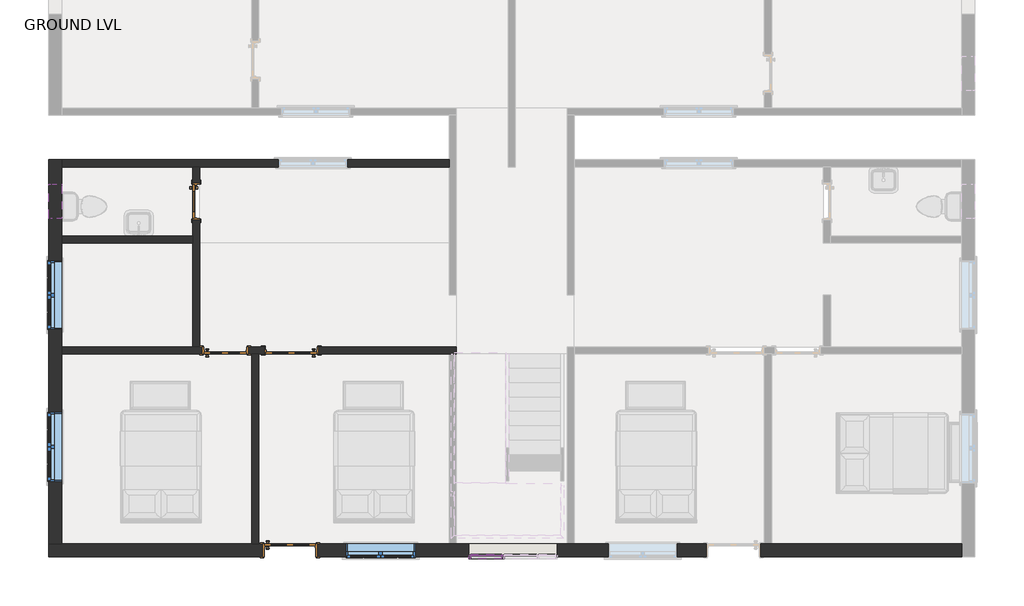
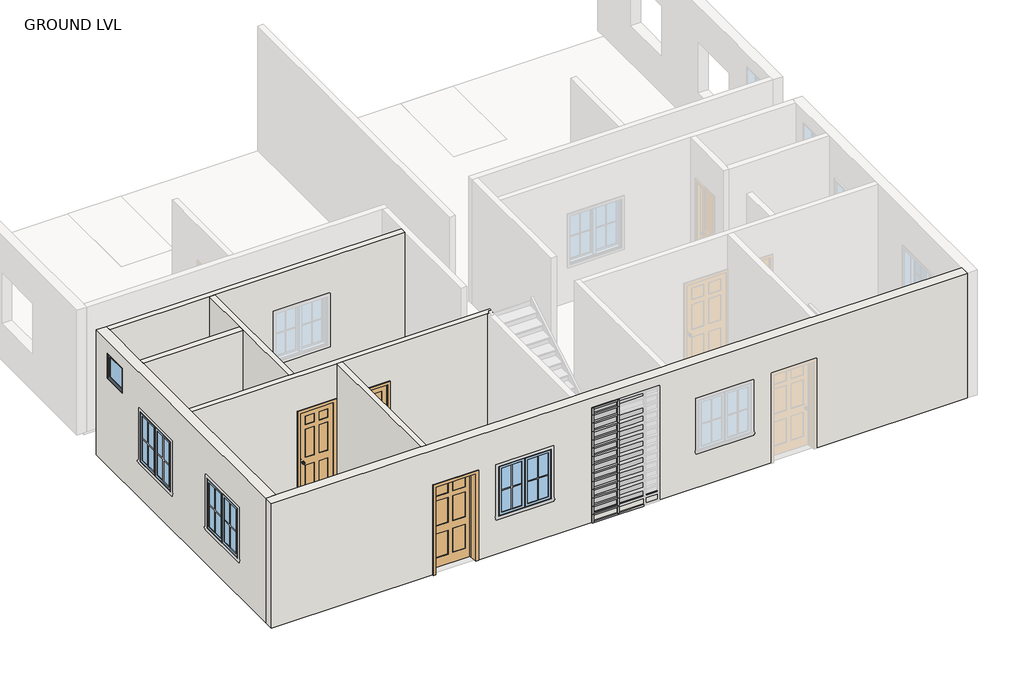
# One storey, part 1 of 4: 44 members, 27 plates, 7 walls, 4 doors, 4 windows.
"""IFC4 building model written with IfcOpenShell, lengths in millimetres."""

from ifc_helpers import new_model, si_unit, origin, origin_with_axes, place, context, project, spatial, polyline, outline, extrude, faceted_brep, transform, mapped, element, save
from components import door_e337afa5, door_3b50870b, door_d86b6c54, door_03e3dfb5, member_56b223d9, member_a59c64b1, member_fa69921b, member_a67f877f, member_6a7c88b6, member_dc11c383, member_ff422208, system_panel_glazed_844a74e3, system_panel_glazed_a39216e9, system_panel_glazed_b3845325, system_panel_glazed_23b8b45c, system_panel_glazed_26c33eb0, system_panel_glazed_afc0885c, window_80340324, window_9200f5ac

model = new_model("IFC4")

# Units and contexts
model_context = context("Model", 3, world=origin())
ifc_project = project(units=[si_unit("LENGTHUNIT", "METRE", prefix="MILLI")], contexts=[model_context])

# Site, building, storey
site = spatial("IfcSite", under=ifc_project)
building = spatial("IfcBuilding", under=site)
storey = spatial("IfcBuildingStorey", under=building, Name="GROUND LVL", Elevation=0.0)

# Doors
placement = place(None, origin())
door_shape = door_e337afa5(model_context)
element("IfcDoor", 1, ObjectType="Door-Interior-Single-2_Panel-Wood : 24\" x 84\"", at=placement, inside=storey, context=model_context, shape_type="MappedRepresentation", body=[
    mapped(door_shape, transform((-9830.0887331, -1548.6593836, 0.0), x_axis=(0.0, -1.0, 0.0), y_axis=(1.0, 0.0, 0.0), z_axis=(0.0, 0.0, 1.0))),
])
door_2_shape = door_3b50870b(model_context)
element("IfcDoor", 2, ObjectType="Door-Interior-Single-6_Panel-Wood : 30\" x 84\"", at=placement, inside=storey, context=model_context, shape_type="MappedRepresentation", body=[
    mapped(door_2_shape, transform((-9318.9137331, -4180.7343836, 0.0), x_axis=(1.0, 0.0, 0.0), y_axis=(0.0, 1.0, 0.0), z_axis=(0.0, 0.0, 1.0))),
])
door_3_shape = door_d86b6c54(model_context)
element("IfcDoor", 3, ObjectType="Door-Interior-Single-6_Panel-Wood : 36\" x 84\"", at=placement, inside=storey, context=model_context, shape_type="MappedRepresentation", body=[
    mapped(door_3_shape, transform((-8175.9137331, -7704.9843836, 0.0), x_axis=(1.0, 0.0, 0.0), y_axis=(0.0, 1.0, 0.0), z_axis=(0.0, 0.0, 1.0))),
])
door_4_shape = door_03e3dfb5(model_context)
element("IfcDoor", 4, ObjectType="Door-Interior-Single-6_Panel-Wood : 36\" x 84\"", at=placement, inside=storey, context=model_context, shape_type="MappedRepresentation", body=[
    mapped(door_4_shape, transform((-8150.5137331, -4180.7343836, 0.0), x_axis=(-1.0, 0.0, 0.0), y_axis=(0.0, -1.0, 0.0), z_axis=(0.0, 0.0, 1.0))),
])

# Members
member_shape = member_56b223d9(model_context)
element("IfcMember", 5, ObjectType="Rectangular Mullion : 1.5\" x 2.5\" rectangular", at=placement, inside=storey, context=model_context, shape_type="MappedRepresentation", body=[
    mapped(member_shape, transform((-4416.6334597, -7822.4593836, 0.0), x_axis=(1.0, 0.0, 0.0), y_axis=(0.0, -1.0, 0.0), z_axis=(0.0, 0.0, -1.0))),
])
element("IfcMember", 6, ObjectType="Rectangular Mullion : 1.5\" x 2.5\" rectangular", at=placement, inside=storey, context=model_context, shape_type="MappedRepresentation", body=[
    mapped(member_shape, transform((-4416.6334597, -7822.4593836, 203.2), x_axis=(1.0, 0.0, 0.0), y_axis=(0.0, -1.0, 0.0), z_axis=(0.0, 0.0, -1.0))),
])
element("IfcMember", 7, ObjectType="Rectangular Mullion : 1.5\" x 2.5\" rectangular", at=placement, inside=storey, context=model_context, shape_type="MappedRepresentation", body=[
    mapped(member_shape, transform((-4416.6334597, -7822.4593836, 406.4), x_axis=(1.0, 0.0, 0.0), y_axis=(0.0, -1.0, 0.0), z_axis=(0.0, 0.0, -1.0))),
])
element("IfcMember", 8, ObjectType="Rectangular Mullion : 1.5\" x 2.5\" rectangular", at=placement, inside=storey, context=model_context, shape_type="MappedRepresentation", body=[
    mapped(member_shape, transform((-4416.6334597, -7822.4593836, 609.6), x_axis=(1.0, 0.0, 0.0), y_axis=(0.0, -1.0, 0.0), z_axis=(0.0, 0.0, -1.0))),
])
element("IfcMember", 9, ObjectType="Rectangular Mullion : 1.5\" x 2.5\" rectangular", at=placement, inside=storey, context=model_context, shape_type="MappedRepresentation", body=[
    mapped(member_shape, transform((-4416.6334597, -7822.4593836, 812.8), x_axis=(1.0, 0.0, 0.0), y_axis=(0.0, -1.0, 0.0), z_axis=(0.0, 0.0, -1.0))),
])
element("IfcMember", 10, ObjectType="Rectangular Mullion : 1.5\" x 2.5\" rectangular", at=placement, inside=storey, context=model_context, shape_type="MappedRepresentation", body=[
    mapped(member_shape, transform((-4416.6334597, -7822.4593836, 1016.0), x_axis=(1.0, 0.0, 0.0), y_axis=(0.0, -1.0, 0.0), z_axis=(0.0, 0.0, -1.0))),
])
element("IfcMember", 11, ObjectType="Rectangular Mullion : 1.5\" x 2.5\" rectangular", at=placement, inside=storey, context=model_context, shape_type="MappedRepresentation", body=[
    mapped(member_shape, transform((-4416.6334597, -7822.4593836, 1219.2), x_axis=(1.0, 0.0, 0.0), y_axis=(0.0, -1.0, 0.0), z_axis=(0.0, 0.0, -1.0))),
])
element("IfcMember", 12, ObjectType="Rectangular Mullion : 1.5\" x 2.5\" rectangular", at=placement, inside=storey, context=model_context, shape_type="MappedRepresentation", body=[
    mapped(member_shape, transform((-4416.6334597, -7822.4593836, 1422.4), x_axis=(1.0, 0.0, 0.0), y_axis=(0.0, -1.0, 0.0), z_axis=(0.0, 0.0, -1.0))),
])
element("IfcMember", 13, ObjectType="Rectangular Mullion : 1.5\" x 2.5\" rectangular", at=placement, inside=storey, context=model_context, shape_type="MappedRepresentation", body=[
    mapped(member_shape, transform((-4416.6334597, -7822.4593836, 1625.6), x_axis=(1.0, 0.0, 0.0), y_axis=(0.0, -1.0, 0.0), z_axis=(0.0, 0.0, -1.0))),
])
element("IfcMember", 14, ObjectType="Rectangular Mullion : 1.5\" x 2.5\" rectangular", at=placement, inside=storey, context=model_context, shape_type="MappedRepresentation", body=[
    mapped(member_shape, transform((-4416.6334597, -7822.4593836, 1828.8), x_axis=(1.0, 0.0, 0.0), y_axis=(0.0, -1.0, 0.0), z_axis=(0.0, 0.0, -1.0))),
])
element("IfcMember", 15, ObjectType="Rectangular Mullion : 1.5\" x 2.5\" rectangular", at=placement, inside=storey, context=model_context, shape_type="MappedRepresentation", body=[
    mapped(member_shape, transform((-4416.6334597, -7822.4593836, 2032.0), x_axis=(1.0, 0.0, 0.0), y_axis=(0.0, -1.0, 0.0), z_axis=(0.0, 0.0, -1.0))),
])
element("IfcMember", 16, ObjectType="Rectangular Mullion : 1.5\" x 2.5\" rectangular", at=placement, inside=storey, context=model_context, shape_type="MappedRepresentation", body=[
    mapped(member_shape, transform((-4416.6334597, -7822.4593836, 2235.2), x_axis=(1.0, 0.0, 0.0), y_axis=(0.0, -1.0, 0.0), z_axis=(0.0, 0.0, -1.0))),
])
element("IfcMember", 17, ObjectType="Rectangular Mullion : 1.5\" x 2.5\" rectangular", at=placement, inside=storey, context=model_context, shape_type="MappedRepresentation", body=[
    mapped(member_shape, transform((-4416.6334597, -7822.4593836, 2438.4), x_axis=(1.0, 0.0, 0.0), y_axis=(0.0, -1.0, 0.0), z_axis=(0.0, 0.0, -1.0))),
])
member_2_shape = member_a59c64b1(model_context)
element("IfcMember", 18, ObjectType="Rectangular Mullion : 1.5\" x 2.5\" rectangular", at=placement, inside=storey, context=model_context, shape_type="MappedRepresentation", body=[
    mapped(member_2_shape, transform((-4416.6334597, -7822.4593836, 2641.6), x_axis=(1.0, 0.0, 0.0), y_axis=(0.0, -1.0, 0.0), z_axis=(0.0, 0.0, -1.0))),
])
member_3_shape = member_fa69921b(model_context)
element("IfcMember", 19, ObjectType="Rectangular Mullion : 1.5\" x 2.5\" rectangular", at=placement, inside=storey, context=model_context, shape_type="MappedRepresentation", body=[
    mapped(member_3_shape, transform((-4435.6834597, -7822.4593836, 2807.3826151), x_axis=(0.0, 0.0, 1.0), y_axis=(0.0, -1.0, 0.0), z_axis=(1.0, 0.0, 0.0))),
])
element("IfcMember", 20, ObjectType="Rectangular Mullion : 1.5\" x 2.5\" rectangular", at=placement, inside=storey, context=model_context, shape_type="MappedRepresentation", body=[
    mapped(member_3_shape, transform((-4988.13346, -7822.4593836, 0.0), x_axis=(0.0, 0.0, -1.0), y_axis=(0.0, -1.0, 0.0), z_axis=(-1.0, 0.0, 0.0))),
])
member_4_shape = member_a67f877f(model_context)
element("IfcMember", 21, ObjectType="Rectangular Mullion : 1.5\" x 2.5\" rectangular", at=placement, inside=storey, context=model_context, shape_type="MappedRepresentation", body=[
    mapped(member_4_shape, transform((-4397.5834597, -7822.4593836, 0.0), x_axis=(0.0, 0.0, -1.0), y_axis=(0.0, -1.0, 0.0), z_axis=(-1.0, 0.0, 0.0))),
])
member_5_shape = member_6a7c88b6(model_context)
element("IfcMember", 22, ObjectType="Rectangular Mullion : 1.5\" x 2.5\" rectangular", at=placement, inside=storey, context=model_context, shape_type="MappedRepresentation", body=[
    mapped(member_5_shape, transform((-4435.6834597, -7822.4593836, 203.2), x_axis=(0.0, 0.0, 1.0), y_axis=(0.0, -1.0, 0.0), z_axis=(1.0, 0.0, 0.0))),
])
element("IfcMember", 23, ObjectType="Rectangular Mullion : 1.5\" x 2.5\" rectangular", at=placement, inside=storey, context=model_context, shape_type="MappedRepresentation", body=[
    mapped(member_5_shape, transform((-4435.6834597, -7822.4593836, 406.4), x_axis=(0.0, 0.0, 1.0), y_axis=(0.0, -1.0, 0.0), z_axis=(1.0, 0.0, 0.0))),
])
element("IfcMember", 24, ObjectType="Rectangular Mullion : 1.5\" x 2.5\" rectangular", at=placement, inside=storey, context=model_context, shape_type="MappedRepresentation", body=[
    mapped(member_5_shape, transform((-4435.6834597, -7822.4593836, 609.6), x_axis=(0.0, 0.0, 1.0), y_axis=(0.0, -1.0, 0.0), z_axis=(1.0, 0.0, 0.0))),
])
element("IfcMember", 25, ObjectType="Rectangular Mullion : 1.5\" x 2.5\" rectangular", at=placement, inside=storey, context=model_context, shape_type="MappedRepresentation", body=[
    mapped(member_5_shape, transform((-4435.6834597, -7822.4593836, 812.8), x_axis=(0.0, 0.0, 1.0), y_axis=(0.0, -1.0, 0.0), z_axis=(1.0, 0.0, 0.0))),
])
element("IfcMember", 26, ObjectType="Rectangular Mullion : 1.5\" x 2.5\" rectangular", at=placement, inside=storey, context=model_context, shape_type="MappedRepresentation", body=[
    mapped(member_5_shape, transform((-4435.6834597, -7822.4593836, 1016.0), x_axis=(0.0, 0.0, 1.0), y_axis=(0.0, -1.0, 0.0), z_axis=(1.0, 0.0, 0.0))),
])
element("IfcMember", 27, ObjectType="Rectangular Mullion : 1.5\" x 2.5\" rectangular", at=placement, inside=storey, context=model_context, shape_type="MappedRepresentation", body=[
    mapped(member_5_shape, transform((-4435.6834597, -7822.4593836, 1219.2), x_axis=(0.0, 0.0, 1.0), y_axis=(0.0, -1.0, 0.0), z_axis=(1.0, 0.0, 0.0))),
])
element("IfcMember", 28, ObjectType="Rectangular Mullion : 1.5\" x 2.5\" rectangular", at=placement, inside=storey, context=model_context, shape_type="MappedRepresentation", body=[
    mapped(member_5_shape, transform((-4435.6834597, -7822.4593836, 1422.4), x_axis=(0.0, 0.0, 1.0), y_axis=(0.0, -1.0, 0.0), z_axis=(1.0, 0.0, 0.0))),
])
element("IfcMember", 29, ObjectType="Rectangular Mullion : 1.5\" x 2.5\" rectangular", at=placement, inside=storey, context=model_context, shape_type="MappedRepresentation", body=[
    mapped(member_5_shape, transform((-4435.6834597, -7822.4593836, 1625.6), x_axis=(0.0, 0.0, 1.0), y_axis=(0.0, -1.0, 0.0), z_axis=(1.0, 0.0, 0.0))),
])
element("IfcMember", 30, ObjectType="Rectangular Mullion : 1.5\" x 2.5\" rectangular", at=placement, inside=storey, context=model_context, shape_type="MappedRepresentation", body=[
    mapped(member_5_shape, transform((-4435.6834597, -7822.4593836, 1828.8), x_axis=(0.0, 0.0, 1.0), y_axis=(0.0, -1.0, 0.0), z_axis=(1.0, 0.0, 0.0))),
])
element("IfcMember", 31, ObjectType="Rectangular Mullion : 1.5\" x 2.5\" rectangular", at=placement, inside=storey, context=model_context, shape_type="MappedRepresentation", body=[
    mapped(member_5_shape, transform((-4435.6834597, -7822.4593836, 2032.0), x_axis=(0.0, 0.0, 1.0), y_axis=(0.0, -1.0, 0.0), z_axis=(1.0, 0.0, 0.0))),
])
element("IfcMember", 32, ObjectType="Rectangular Mullion : 1.5\" x 2.5\" rectangular", at=placement, inside=storey, context=model_context, shape_type="MappedRepresentation", body=[
    mapped(member_5_shape, transform((-4435.6834597, -7822.4593836, 2235.2), x_axis=(0.0, 0.0, 1.0), y_axis=(0.0, -1.0, 0.0), z_axis=(1.0, 0.0, 0.0))),
])
element("IfcMember", 33, ObjectType="Rectangular Mullion : 1.5\" x 2.5\" rectangular", at=placement, inside=storey, context=model_context, shape_type="MappedRepresentation", body=[
    mapped(member_5_shape, transform((-4435.6834597, -7822.4593836, 2438.4), x_axis=(0.0, 0.0, 1.0), y_axis=(0.0, -1.0, 0.0), z_axis=(1.0, 0.0, 0.0))),
])
element("IfcMember", 34, ObjectType="Rectangular Mullion : 1.5\" x 2.5\" rectangular", at=placement, inside=storey, context=model_context, shape_type="MappedRepresentation", body=[
    mapped(member_5_shape, transform((-4435.6834597, -7822.4593836, 2641.6), x_axis=(0.0, 0.0, 1.0), y_axis=(0.0, -1.0, 0.0), z_axis=(1.0, 0.0, 0.0))),
])
member_6_shape = member_dc11c383(model_context)
element("IfcMember", 35, ObjectType="Rectangular Mullion : 1.5\" x 2.5\" rectangular", at=placement, inside=storey, context=model_context, shape_type="MappedRepresentation", body=[
    mapped(member_6_shape, transform((-5026.23346, -7822.4593836, 2807.3826151), x_axis=(-1.0, 0.0, 0.0), y_axis=(0.0, -1.0, 0.0), z_axis=(0.0, 0.0, 1.0))),
])
member_7_shape = member_ff422208(model_context)
element("IfcMember", 36, ObjectType="Rectangular Mullion : 1.5\" x 2.5\" rectangular", at=placement, inside=storey, context=model_context, shape_type="MappedRepresentation", body=[
    mapped(member_7_shape, transform((-5026.23346, -7822.4593836, 203.2), x_axis=(-1.0, 0.0, 0.0), y_axis=(0.0, -1.0, 0.0), z_axis=(0.0, 0.0, 1.0))),
])
element("IfcMember", 37, ObjectType="Rectangular Mullion : 1.5\" x 2.5\" rectangular", at=placement, inside=storey, context=model_context, shape_type="MappedRepresentation", body=[
    mapped(member_7_shape, transform((-5026.23346, -7822.4593836, 406.4), x_axis=(-1.0, 0.0, 0.0), y_axis=(0.0, -1.0, 0.0), z_axis=(0.0, 0.0, 1.0))),
])
element("IfcMember", 38, ObjectType="Rectangular Mullion : 1.5\" x 2.5\" rectangular", at=placement, inside=storey, context=model_context, shape_type="MappedRepresentation", body=[
    mapped(member_7_shape, transform((-5026.23346, -7822.4593836, 609.6), x_axis=(-1.0, 0.0, 0.0), y_axis=(0.0, -1.0, 0.0), z_axis=(0.0, 0.0, 1.0))),
])
element("IfcMember", 39, ObjectType="Rectangular Mullion : 1.5\" x 2.5\" rectangular", at=placement, inside=storey, context=model_context, shape_type="MappedRepresentation", body=[
    mapped(member_7_shape, transform((-5026.23346, -7822.4593836, 812.8), x_axis=(-1.0, 0.0, 0.0), y_axis=(0.0, -1.0, 0.0), z_axis=(0.0, 0.0, 1.0))),
])
element("IfcMember", 40, ObjectType="Rectangular Mullion : 1.5\" x 2.5\" rectangular", at=placement, inside=storey, context=model_context, shape_type="MappedRepresentation", body=[
    mapped(member_7_shape, transform((-5026.23346, -7822.4593836, 1016.0), x_axis=(-1.0, 0.0, 0.0), y_axis=(0.0, -1.0, 0.0), z_axis=(0.0, 0.0, 1.0))),
])
element("IfcMember", 41, ObjectType="Rectangular Mullion : 1.5\" x 2.5\" rectangular", at=placement, inside=storey, context=model_context, shape_type="MappedRepresentation", body=[
    mapped(member_7_shape, transform((-5026.23346, -7822.4593836, 1219.2), x_axis=(-1.0, 0.0, 0.0), y_axis=(0.0, -1.0, 0.0), z_axis=(0.0, 0.0, 1.0))),
])
element("IfcMember", 42, ObjectType="Rectangular Mullion : 1.5\" x 2.5\" rectangular", at=placement, inside=storey, context=model_context, shape_type="MappedRepresentation", body=[
    mapped(member_7_shape, transform((-5026.23346, -7822.4593836, 1422.4), x_axis=(-1.0, 0.0, 0.0), y_axis=(0.0, -1.0, 0.0), z_axis=(0.0, 0.0, 1.0))),
])
element("IfcMember", 43, ObjectType="Rectangular Mullion : 1.5\" x 2.5\" rectangular", at=placement, inside=storey, context=model_context, shape_type="MappedRepresentation", body=[
    mapped(member_7_shape, transform((-5026.23346, -7822.4593836, 1625.6), x_axis=(-1.0, 0.0, 0.0), y_axis=(0.0, -1.0, 0.0), z_axis=(0.0, 0.0, 1.0))),
])
element("IfcMember", 44, ObjectType="Rectangular Mullion : 1.5\" x 2.5\" rectangular", at=placement, inside=storey, context=model_context, shape_type="MappedRepresentation", body=[
    mapped(member_7_shape, transform((-5026.23346, -7822.4593836, 1828.8), x_axis=(-1.0, 0.0, 0.0), y_axis=(0.0, -1.0, 0.0), z_axis=(0.0, 0.0, 1.0))),
])
element("IfcMember", 45, ObjectType="Rectangular Mullion : 1.5\" x 2.5\" rectangular", at=placement, inside=storey, context=model_context, shape_type="MappedRepresentation", body=[
    mapped(member_7_shape, transform((-5026.23346, -7822.4593836, 2032.0), x_axis=(-1.0, 0.0, 0.0), y_axis=(0.0, -1.0, 0.0), z_axis=(0.0, 0.0, 1.0))),
])
element("IfcMember", 46, ObjectType="Rectangular Mullion : 1.5\" x 2.5\" rectangular", at=placement, inside=storey, context=model_context, shape_type="MappedRepresentation", body=[
    mapped(member_7_shape, transform((-5026.23346, -7822.4593836, 2235.2), x_axis=(-1.0, 0.0, 0.0), y_axis=(0.0, -1.0, 0.0), z_axis=(0.0, 0.0, 1.0))),
])
element("IfcMember", 47, ObjectType="Rectangular Mullion : 1.5\" x 2.5\" rectangular", at=placement, inside=storey, context=model_context, shape_type="MappedRepresentation", body=[
    mapped(member_7_shape, transform((-5026.23346, -7822.4593836, 2438.4), x_axis=(-1.0, 0.0, 0.0), y_axis=(0.0, -1.0, 0.0), z_axis=(0.0, 0.0, 1.0))),
])
element("IfcMember", 48, ObjectType="Rectangular Mullion : 1.5\" x 2.5\" rectangular", at=placement, inside=storey, context=model_context, shape_type="MappedRepresentation", body=[
    mapped(member_7_shape, transform((-5026.23346, -7822.4593836, 2641.6), x_axis=(-1.0, 0.0, 0.0), y_axis=(0.0, -1.0, 0.0), z_axis=(0.0, 0.0, 1.0))),
])

# Plates
system_panel_glazed_shape = system_panel_glazed_844a74e3(model_context)
element("IfcPlate", 49, ObjectType="System Panel : Glazed", at=placement, inside=storey, context=model_context, shape_type="MappedRepresentation", body=[
    mapped(system_panel_glazed_shape, transform((-4711.9084599, -7822.4593836, 38.1), x_axis=(1.0, 0.0, 0.0), y_axis=(0.0, 1.0, 0.0), z_axis=(0.0, 0.0, 1.0))),
])
system_panel_glazed_2_shape = system_panel_glazed_a39216e9(model_context)
element("IfcPlate", 50, ObjectType="System Panel : Glazed", at=placement, inside=storey, context=model_context, shape_type="MappedRepresentation", body=[
    mapped(system_panel_glazed_2_shape, transform((-4111.8334597, -7822.4593836, 38.1), x_axis=(1.0, 0.0, 0.0), y_axis=(0.0, 1.0, 0.0), z_axis=(0.0, 0.0, 1.0))),
])
system_panel_glazed_3_shape = system_panel_glazed_b3845325(model_context)
element("IfcPlate", 51, ObjectType="System Panel : Glazed", at=placement, inside=storey, context=model_context, shape_type="MappedRepresentation", body=[
    mapped(system_panel_glazed_3_shape, transform((-4711.9084599, -7822.4593836, 222.25), x_axis=(1.0, 0.0, 0.0), y_axis=(0.0, 1.0, 0.0), z_axis=(0.0, 0.0, 1.0))),
])
element("IfcPlate", 52, ObjectType="System Panel : Glazed", at=placement, inside=storey, context=model_context, shape_type="MappedRepresentation", body=[
    mapped(system_panel_glazed_3_shape, transform((-4711.9084599, -7822.4593836, 425.45), x_axis=(1.0, 0.0, 0.0), y_axis=(0.0, 1.0, 0.0), z_axis=(0.0, 0.0, 1.0))),
])
element("IfcPlate", 53, ObjectType="System Panel : Glazed", at=placement, inside=storey, context=model_context, shape_type="MappedRepresentation", body=[
    mapped(system_panel_glazed_3_shape, transform((-4711.9084599, -7822.4593836, 831.85), x_axis=(1.0, 0.0, 0.0), y_axis=(0.0, 1.0, 0.0), z_axis=(0.0, 0.0, 1.0))),
])
element("IfcPlate", 54, ObjectType="System Panel : Glazed", at=placement, inside=storey, context=model_context, shape_type="MappedRepresentation", body=[
    mapped(system_panel_glazed_3_shape, transform((-4711.9084599, -7822.4593836, 1035.05), x_axis=(1.0, 0.0, 0.0), y_axis=(0.0, 1.0, 0.0), z_axis=(0.0, 0.0, 1.0))),
])
element("IfcPlate", 55, ObjectType="System Panel : Glazed", at=placement, inside=storey, context=model_context, shape_type="MappedRepresentation", body=[
    mapped(system_panel_glazed_3_shape, transform((-4711.9084599, -7822.4593836, 1441.45), x_axis=(1.0, 0.0, 0.0), y_axis=(0.0, 1.0, 0.0), z_axis=(0.0, 0.0, 1.0))),
])
element("IfcPlate", 56, ObjectType="System Panel : Glazed", at=placement, inside=storey, context=model_context, shape_type="MappedRepresentation", body=[
    mapped(system_panel_glazed_3_shape, transform((-4711.9084599, -7822.4593836, 1644.65), x_axis=(1.0, 0.0, 0.0), y_axis=(0.0, 1.0, 0.0), z_axis=(0.0, 0.0, 1.0))),
])
element("IfcPlate", 57, ObjectType="System Panel : Glazed", at=placement, inside=storey, context=model_context, shape_type="MappedRepresentation", body=[
    mapped(system_panel_glazed_3_shape, transform((-4711.9084599, -7822.4593836, 2051.05), x_axis=(1.0, 0.0, 0.0), y_axis=(0.0, 1.0, 0.0), z_axis=(0.0, 0.0, 1.0))),
])
element("IfcPlate", 58, ObjectType="System Panel : Glazed", at=placement, inside=storey, context=model_context, shape_type="MappedRepresentation", body=[
    mapped(system_panel_glazed_3_shape, transform((-4711.9084599, -7822.4593836, 2254.25), x_axis=(1.0, 0.0, 0.0), y_axis=(0.0, 1.0, 0.0), z_axis=(0.0, 0.0, 1.0))),
])
element("IfcPlate", 59, ObjectType="System Panel : Glazed", at=placement, inside=storey, context=model_context, shape_type="MappedRepresentation", body=[
    mapped(system_panel_glazed_3_shape, transform((-4711.9084599, -7822.4593836, 628.65), x_axis=(1.0, 0.0, 0.0), y_axis=(0.0, 1.0, 0.0), z_axis=(0.0, 0.0, 1.0))),
])
element("IfcPlate", 60, ObjectType="System Panel : Glazed", at=placement, inside=storey, context=model_context, shape_type="MappedRepresentation", body=[
    mapped(system_panel_glazed_3_shape, transform((-4711.9084599, -7822.4593836, 1238.25), x_axis=(1.0, 0.0, 0.0), y_axis=(0.0, 1.0, 0.0), z_axis=(0.0, 0.0, 1.0))),
])
element("IfcPlate", 61, ObjectType="System Panel : Glazed", at=placement, inside=storey, context=model_context, shape_type="MappedRepresentation", body=[
    mapped(system_panel_glazed_3_shape, transform((-4711.9084599, -7822.4593836, 1847.85), x_axis=(1.0, 0.0, 0.0), y_axis=(0.0, 1.0, 0.0), z_axis=(0.0, 0.0, 1.0))),
])
element("IfcPlate", 62, ObjectType="System Panel : Glazed", at=placement, inside=storey, context=model_context, shape_type="MappedRepresentation", body=[
    mapped(system_panel_glazed_3_shape, transform((-4711.9084599, -7822.4593836, 2457.45), x_axis=(1.0, 0.0, 0.0), y_axis=(0.0, 1.0, 0.0), z_axis=(0.0, 0.0, 1.0))),
])
system_panel_glazed_4_shape = system_panel_glazed_23b8b45c(model_context)
element("IfcPlate", 63, ObjectType="System Panel : Glazed", at=placement, inside=storey, context=model_context, shape_type="MappedRepresentation", body=[
    mapped(system_panel_glazed_4_shape, transform((-4111.8334597, -7822.4593836, 222.25), x_axis=(1.0, 0.0, 0.0), y_axis=(0.0, 1.0, 0.0), z_axis=(0.0, 0.0, 1.0))),
])
element("IfcPlate", 64, ObjectType="System Panel : Glazed", at=placement, inside=storey, context=model_context, shape_type="MappedRepresentation", body=[
    mapped(system_panel_glazed_4_shape, transform((-4111.8334597, -7822.4593836, 425.45), x_axis=(1.0, 0.0, 0.0), y_axis=(0.0, 1.0, 0.0), z_axis=(0.0, 0.0, 1.0))),
])
element("IfcPlate", 65, ObjectType="System Panel : Glazed", at=placement, inside=storey, context=model_context, shape_type="MappedRepresentation", body=[
    mapped(system_panel_glazed_4_shape, transform((-4111.8334597, -7822.4593836, 831.85), x_axis=(1.0, 0.0, 0.0), y_axis=(0.0, 1.0, 0.0), z_axis=(0.0, 0.0, 1.0))),
])
element("IfcPlate", 66, ObjectType="System Panel : Glazed", at=placement, inside=storey, context=model_context, shape_type="MappedRepresentation", body=[
    mapped(system_panel_glazed_4_shape, transform((-4111.8334597, -7822.4593836, 1035.05), x_axis=(1.0, 0.0, 0.0), y_axis=(0.0, 1.0, 0.0), z_axis=(0.0, 0.0, 1.0))),
])
element("IfcPlate", 67, ObjectType="System Panel : Glazed", at=placement, inside=storey, context=model_context, shape_type="MappedRepresentation", body=[
    mapped(system_panel_glazed_4_shape, transform((-4111.8334597, -7822.4593836, 1441.45), x_axis=(1.0, 0.0, 0.0), y_axis=(0.0, 1.0, 0.0), z_axis=(0.0, 0.0, 1.0))),
])
element("IfcPlate", 68, ObjectType="System Panel : Glazed", at=placement, inside=storey, context=model_context, shape_type="MappedRepresentation", body=[
    mapped(system_panel_glazed_4_shape, transform((-4111.8334597, -7822.4593836, 1644.65), x_axis=(1.0, 0.0, 0.0), y_axis=(0.0, 1.0, 0.0), z_axis=(0.0, 0.0, 1.0))),
])
element("IfcPlate", 69, ObjectType="System Panel : Glazed", at=placement, inside=storey, context=model_context, shape_type="MappedRepresentation", body=[
    mapped(system_panel_glazed_4_shape, transform((-4111.8334597, -7822.4593836, 2051.05), x_axis=(1.0, 0.0, 0.0), y_axis=(0.0, 1.0, 0.0), z_axis=(0.0, 0.0, 1.0))),
])
element("IfcPlate", 70, ObjectType="System Panel : Glazed", at=placement, inside=storey, context=model_context, shape_type="MappedRepresentation", body=[
    mapped(system_panel_glazed_4_shape, transform((-4111.8334597, -7822.4593836, 2254.25), x_axis=(1.0, 0.0, 0.0), y_axis=(0.0, 1.0, 0.0), z_axis=(0.0, 0.0, 1.0))),
])
element("IfcPlate", 71, ObjectType="System Panel : Glazed", at=placement, inside=storey, context=model_context, shape_type="MappedRepresentation", body=[
    mapped(system_panel_glazed_4_shape, transform((-4111.8334597, -7822.4593836, 628.65), x_axis=(1.0, 0.0, 0.0), y_axis=(0.0, 1.0, 0.0), z_axis=(0.0, 0.0, 1.0))),
])
element("IfcPlate", 72, ObjectType="System Panel : Glazed", at=placement, inside=storey, context=model_context, shape_type="MappedRepresentation", body=[
    mapped(system_panel_glazed_4_shape, transform((-4111.8334597, -7822.4593836, 1238.25), x_axis=(1.0, 0.0, 0.0), y_axis=(0.0, 1.0, 0.0), z_axis=(0.0, 0.0, 1.0))),
])
element("IfcPlate", 73, ObjectType="System Panel : Glazed", at=placement, inside=storey, context=model_context, shape_type="MappedRepresentation", body=[
    mapped(system_panel_glazed_4_shape, transform((-4111.8334597, -7822.4593836, 1847.85), x_axis=(1.0, 0.0, 0.0), y_axis=(0.0, 1.0, 0.0), z_axis=(0.0, 0.0, 1.0))),
])
system_panel_glazed_5_shape = system_panel_glazed_26c33eb0(model_context)
element("IfcPlate", 74, ObjectType="System Panel : Glazed", at=placement, inside=storey, context=model_context, shape_type="MappedRepresentation", body=[
    mapped(system_panel_glazed_5_shape, transform((-4711.9084599, -7822.4593836, 2660.65), x_axis=(1.0, 0.0, 0.0), y_axis=(0.0, 1.0, 0.0), z_axis=(0.0, 0.0, 1.0))),
])
system_panel_glazed_6_shape = system_panel_glazed_afc0885c(model_context)
element("IfcPlate", 75, ObjectType="System Panel : Glazed", at=placement, inside=storey, context=model_context, shape_type="MappedRepresentation", body=[
    mapped(system_panel_glazed_6_shape, transform((-4111.8334597, -7822.4593836, 2660.65), x_axis=(1.0, 0.0, 0.0), y_axis=(0.0, 1.0, 0.0), z_axis=(0.0, 0.0, 1.0))),
])

# Walls
element("IfcWall", 76, ObjectType="Inner Wall 5\"", at=placement, inside=storey, context=model_context, shape_type="Brep", body=[
    faceted_brep([(-12201.8137331, -939.0593836, 0.0), (-9890.4137331, -939.0593836, 0.0), (-9763.4137331, -939.0593836, 0.0), (-5369.2137331, -939.0593836, 0.0), (-5369.2137331, -939.0593836, 3048.0), (-9763.4137331, -939.0593836, 3048.0), (-9890.4137331, -939.0593836, 3048.0), (-12201.8137331, -939.0593836, 3048.0), (-7159.9137331, -939.0593836, 2133.6), (-7159.9137331, -939.0593836, 914.4), (-8379.1137331, -939.0593836, 914.4), (-8379.1137331, -939.0593836, 2133.6), (-12201.8137331, -812.0593836, 0.0), (-12201.8137331, -812.0593836, 3048.0), (-5369.2137331, -812.0593836, 3048.0), (-5369.2137331, -812.0593836, 0.0), (-7159.9137331, -812.0593836, 2133.6), (-8379.1137331, -812.0593836, 2133.6), (-8379.1137331, -812.0593836, 914.4), (-7159.9137331, -812.0593836, 914.4)], [[[0, 1, 2, 3, 4, 5, 6, 7], [8, 9, 10, 11]], [[12, 13, 14, 15], [16, 17, 18, 19]], [[3, 2, 1, 0, 12, 15]], [[0, 7, 13, 12]], [[4, 3, 15, 14]], [[9, 8, 16, 19]], [[10, 9, 19, 18]], [[11, 10, 18, 17]], [[8, 11, 17, 16]], [[7, 6, 5, 4, 14, 13]]]),
])
element("IfcWall", 77, ObjectType="Inner Wall 5\"", at=placement, inside=storey, context=model_context, shape_type="SweptSolid", body=[
    extrude(outline(polyline([(-8722.0137331, -4241.0593836), (-8722.0137331, -7593.8593836), (-8849.0137331, -7593.8593836), (-8849.0137331, -4241.0593836), (-8722.0137331, -4241.0593836)])), origin_with_axes(), (0.0, 0.0, 1.0), 3048.0),
])
element("IfcWall", 78, ObjectType="Inner Wall 5\"", at=placement, inside=storey, context=model_context, shape_type="Brep", body=[
    faceted_brep([(-12201.8137331, -4114.0593836, 0.0), (-12201.8137331, -4114.0593836, 3048.0), (-9890.4137331, -4114.0593836, 3048.0), (-9763.4137331, -4114.0593836, 3048.0), (-5242.2137331, -4114.0593836, 3048.0), (-5242.2137331, -4114.0593836, 0.0), (-7667.9137331, -4114.0593836, 0.0), (-7667.9137331, -4114.0593836, 2159.0), (-8633.1137331, -4114.0593836, 2159.0), (-8633.1137331, -4114.0593836, 0.0), (-8912.5137331, -4114.0593836, 0.0), (-8912.5137331, -4114.0593836, 2159.0), (-9725.3137331, -4114.0593836, 2159.0), (-9725.3137331, -4114.0593836, 0.0), (-9763.4137331, -4114.0593836, 0.0), (-9890.4137331, -4114.0593836, 0.0), (-12201.8137331, -4241.0593836, 3048.0), (-12201.8137331, -4241.0593836, 0.0), (-9725.3137331, -4241.0593836, 0.0), (-9725.3137331, -4241.0593836, 2159.0), (-8912.5137331, -4241.0593836, 2159.0), (-8912.5137331, -4241.0593836, 0.0), (-8849.0137331, -4241.0593836, 0.0), (-8722.0137331, -4241.0593836, 0.0), (-8633.1137331, -4241.0593836, 0.0), (-8633.1137331, -4241.0593836, 2159.0), (-7667.9137331, -4241.0593836, 2159.0), (-7667.9137331, -4241.0593836, 0.0), (-5369.2137331, -4241.0593836, 0.0), (-5242.2137331, -4241.0593836, 0.0), (-5242.2137331, -4241.0593836, 3048.0), (-5369.2137331, -4241.0593836, 3048.0), (-8722.0137331, -4241.0593836, 3048.0), (-8849.0137331, -4241.0593836, 3048.0)], [[[0, 1, 2, 3, 4, 5, 6, 7, 8, 9, 10, 11, 12, 13, 14, 15]], [[16, 17, 18, 19, 20, 21, 22, 23, 24, 25, 26, 27, 28, 29, 30, 31, 32, 33]], [[17, 0, 15, 14, 13, 18]], [[5, 29, 28, 27, 6]], [[21, 10, 9, 24, 23, 22]], [[1, 0, 17, 16]], [[5, 4, 30, 29]], [[11, 10, 21, 20]], [[12, 11, 20, 19]], [[13, 12, 19, 18]], [[8, 25, 24, 9]], [[25, 8, 7, 26]], [[26, 7, 6, 27]], [[4, 3, 2, 1, 16, 33, 32, 31, 30]]]),
])
element("IfcWall", 79, ObjectType="Inner Wall 5\"", at=placement, inside=storey, context=model_context, shape_type="Brep", body=[
    faceted_brep([(-9763.4137331, -4114.0593836, 3048.0), (-9763.4137331, -4114.0593836, 0.0), (-9763.4137331, -1878.8593836, 0.0), (-9763.4137331, -1878.8593836, 2159.0), (-9763.4137331, -1218.4593836, 2159.0), (-9763.4137331, -1218.4593836, 0.0), (-9763.4137331, -939.0593836, 0.0), (-9763.4137331, -939.0593836, 3048.0), (-9890.4137331, -4114.0593836, 0.0), (-9890.4137331, -4114.0593836, 3048.0), (-9890.4137331, -2285.2593836, 3048.0), (-9890.4137331, -2158.2593836, 3048.0), (-9890.4137331, -939.0593836, 3048.0), (-9890.4137331, -939.0593836, 0.0), (-9890.4137331, -1218.4593836, 0.0), (-9890.4137331, -1218.4593836, 2159.0), (-9890.4137331, -1878.8593836, 2159.0), (-9890.4137331, -1878.8593836, 0.0), (-9890.4137331, -2158.2593836, 0.0), (-9890.4137331, -2285.2593836, 0.0)], [[[0, 1, 2, 3, 4, 5, 6, 7]], [[8, 9, 10, 11, 12, 13, 14, 15, 16, 17, 18, 19]], [[1, 8, 19, 18, 17, 2]], [[13, 6, 5, 14]], [[1, 0, 9, 8]], [[7, 6, 13, 12]], [[16, 3, 2, 17]], [[3, 16, 15, 4]], [[4, 15, 14, 5]], [[0, 7, 12, 11, 10, 9]]]),
])
element("IfcWall", 80, ObjectType="Inner Wall 5\"", at=placement, inside=storey, context=model_context, shape_type="SweptSolid", body=[
    extrude(outline(polyline([(-12201.8137331, -2158.2593836), (-9890.4137331, -2158.2593836), (-9890.4137331, -2285.2593836), (-12201.8137331, -2285.2593836), (-12201.8137331, -2158.2593836)])), origin_with_axes(), (0.0, 0.0, 1.0), 3048.0),
])
element("IfcWall", 81, ObjectType="outer wall 9\"", at=placement, inside=storey, context=model_context, shape_type="Brep", body=[
    faceted_brep([(-12430.4137331, -7822.4593836, 3048.0), (-12430.4137331, -7822.4593836, 0.0), (-8658.5137331, -7822.4593836, 0.0), (-8658.5137331, -7822.4593836, 2159.0), (-7693.3137331, -7822.4593836, 2159.0), (-7693.3137331, -7822.4593836, 0.0), (-835.3137331, -7822.4593836, 0.0), (-835.3137331, -7822.4593836, 2159.0), (129.8862669, -7822.4593836, 2159.0), (129.8862669, -7822.4593836, 0.0), (3673.1862669, -7822.4593836, 0.0), (3673.1862669, -7822.4593836, 3048.0), (-3159.4137331, -7822.4593836, 3048.0), (-5369.2137331, -7822.4593836, 3048.0), (-2562.5137331, -7822.4593836, 2133.6), (-1343.3137331, -7822.4593836, 2133.6), (-1343.3137331, -7822.4593836, 914.4), (-2562.5137331, -7822.4593836, 914.4), (-7185.3137331, -7822.4593836, 2133.6), (-5966.1137331, -7822.4593836, 2133.6), (-5966.1137331, -7822.4593836, 914.4), (-7185.3137331, -7822.4593836, 914.4), (-5026.23346, -7822.4593836, 2807.3826151), (-3461.6513929, -7822.4593836, 2807.3826151), (-3461.6513929, -7822.4593836, 234.5143269), (-5026.23346, -7822.4593836, 234.5143269), (-12430.4137331, -7593.8593836, 3048.0), (-12201.8137331, -7593.8593836, 3048.0), (-8849.0137331, -7593.8593836, 3048.0), (-8722.0137331, -7593.8593836, 3048.0), (-5369.2137331, -7593.8593836, 3048.0), (-5242.2137331, -7593.8593836, 3048.0), (-3286.4137331, -7593.8593836, 3048.0), (-3159.4137331, -7593.8593836, 3048.0), (193.3862669, -7593.8593836, 3048.0), (320.3862669, -7593.8593836, 3048.0), (3673.1862669, -7593.8593836, 3048.0), (3673.1862669, -7593.8593836, 0.0), (320.3862669, -7593.8593836, 0.0), (193.3862669, -7593.8593836, 0.0), (129.8862669, -7593.8593836, 0.0), (129.8862669, -7593.8593836, 2159.0), (-835.3137331, -7593.8593836, 2159.0), (-835.3137331, -7593.8593836, 0.0), (-3159.4137331, -7593.8593836, 0.0), (-3286.4137331, -7593.8593836, 0.0), (-5242.2137331, -7593.8593836, 0.0), (-5369.2137331, -7593.8593836, 0.0), (-7693.3137331, -7593.8593836, 0.0), (-7693.3137331, -7593.8593836, 2159.0), (-8658.5137331, -7593.8593836, 2159.0), (-8658.5137331, -7593.8593836, 0.0), (-8722.0137331, -7593.8593836, 0.0), (-8849.0137331, -7593.8593836, 0.0), (-12201.8137331, -7593.8593836, 0.0), (-12430.4137331, -7593.8593836, 0.0), (-2562.5137331, -7593.8593836, 2133.6), (-2562.5137331, -7593.8593836, 914.4), (-1343.3137331, -7593.8593836, 914.4), (-1343.3137331, -7593.8593836, 2133.6), (-7185.3137331, -7593.8593836, 2133.6), (-7185.3137331, -7593.8593836, 914.4), (-5966.1137331, -7593.8593836, 914.4), (-5966.1137331, -7593.8593836, 2133.6), (-3461.6513929, -7593.8593836, 2807.3826151), (-5026.23346, -7593.8593836, 2807.3826151), (-5026.23346, -7593.8593836, 234.5143269), (-3461.6513929, -7593.8593836, 234.5143269)], [[[0, 1, 2, 3, 4, 5, 6, 7, 8, 9, 10, 11, 12, 13], [14, 15, 16, 17], [18, 19, 20, 21], [22, 23, 24, 25]], [[26, 27, 28, 29, 30, 31, 32, 33, 34, 35, 36, 37, 38, 39, 40, 41, 42, 43, 44, 45, 46, 47, 48, 49, 50, 51, 52, 53, 54, 55], [56, 57, 58, 59], [60, 61, 62, 63], [64, 65, 66, 67]], [[1, 55, 54, 53, 52, 51, 2]], [[37, 10, 9, 40, 39, 38]], [[5, 48, 47, 46, 45, 44, 43, 6]], [[1, 0, 26, 55]], [[11, 10, 37, 36]], [[4, 49, 48, 5]], [[49, 4, 3, 50]], [[50, 3, 2, 51]], [[42, 7, 6, 43]], [[7, 42, 41, 8]], [[8, 41, 40, 9]], [[57, 56, 14, 17]], [[58, 57, 17, 16]], [[59, 58, 16, 15]], [[56, 59, 15, 14]], [[61, 60, 18, 21]], [[62, 61, 21, 20]], [[63, 62, 20, 19]], [[60, 63, 19, 18]], [[36, 35, 34, 33, 32, 31, 30, 29, 28, 27, 26, 0, 13, 12, 11]], [[22, 65, 64, 23]], [[24, 67, 66, 25]], [[65, 22, 25, 66]], [[23, 64, 67, 24]]]),
])
element("IfcWall", 82, ObjectType="outer wall 9\"", at=placement, inside=storey, context=model_context, shape_type="Brep", body=[
    faceted_brep([(-12430.4137331, -812.0593836, 0.0), (-12430.4137331, -7593.8593836, 0.0), (-12430.4137331, -7593.8593836, 3048.0), (-12430.4137331, -812.0593836, 3048.0), (-12430.4137331, -5269.7593836, 2133.6), (-12430.4137331, -6488.9593836, 2133.6), (-12430.4137331, -6488.9593836, 914.4), (-12430.4137331, -5269.7593836, 914.4), (-12430.4137331, -2590.0593836, 2133.6), (-12430.4137331, -3809.2593836, 2133.6), (-12430.4137331, -3809.2593836, 914.4), (-12430.4137331, -2590.0593836, 914.4), (-12430.4137331, -1243.8593836, 2743.2), (-12430.4137331, -1853.4593836, 2743.2), (-12430.4137331, -1853.4593836, 2133.6), (-12430.4137331, -1243.8593836, 2133.6), (-12201.8137331, -812.0593836, 0.0), (-12201.8137331, -812.0593836, 3048.0), (-12201.8137331, -939.0593836, 3048.0), (-12201.8137331, -2158.2593836, 3048.0), (-12201.8137331, -2285.2593836, 3048.0), (-12201.8137331, -4114.0593836, 3048.0), (-12201.8137331, -4241.0593836, 3048.0), (-12201.8137331, -7593.8593836, 3048.0), (-12201.8137331, -7593.8593836, 0.0), (-12201.8137331, -4241.0593836, 0.0), (-12201.8137331, -4114.0593836, 0.0), (-12201.8137331, -2285.2593836, 0.0), (-12201.8137331, -2158.2593836, 0.0), (-12201.8137331, -939.0593836, 0.0), (-12201.8137331, -5269.7593836, 2133.6), (-12201.8137331, -5269.7593836, 914.4), (-12201.8137331, -6488.9593836, 914.4), (-12201.8137331, -6488.9593836, 2133.6), (-12201.8137331, -2590.0593836, 2133.6), (-12201.8137331, -2590.0593836, 914.4), (-12201.8137331, -3809.2593836, 914.4), (-12201.8137331, -3809.2593836, 2133.6), (-12201.8137331, -1243.8593836, 2743.2), (-12201.8137331, -1243.8593836, 2133.6), (-12201.8137331, -1853.4593836, 2133.6), (-12201.8137331, -1853.4593836, 2743.2)], [[[0, 1, 2, 3], [4, 5, 6, 7], [8, 9, 10, 11], [12, 13, 14, 15]], [[16, 17, 18, 19, 20, 21, 22, 23, 24, 25, 26, 27, 28, 29], [30, 31, 32, 33], [34, 35, 36, 37], [38, 39, 40, 41]], [[1, 0, 16, 29, 28, 27, 26, 25, 24]], [[2, 1, 24, 23]], [[0, 3, 17, 16]], [[31, 30, 4, 7]], [[32, 31, 7, 6]], [[33, 32, 6, 5]], [[30, 33, 5, 4]], [[35, 34, 8, 11]], [[36, 35, 11, 10]], [[37, 36, 10, 9]], [[34, 37, 9, 8]], [[39, 38, 12, 15]], [[40, 39, 15, 14]], [[41, 40, 14, 13]], [[38, 41, 13, 12]], [[3, 2, 23, 22, 21, 20, 19, 18, 17]]]),
])

# Windows
window_shape = window_80340324(model_context)
element("IfcWindow", 83, ObjectType="Fixed : 24\" x 24\"", at=placement, inside=storey, context=model_context, shape_type="MappedRepresentation", body=[
    mapped(window_shape, transform((-12316.1137331, -1510.5593836, 1219.2), x_axis=(0.0, 1.0, 0.0), y_axis=(-1.0, 0.0, 0.0), z_axis=(0.0, 0.0, 1.0))),
])
window_2_shape = window_9200f5ac(model_context)
element("IfcWindow", 84, ObjectType="Window-Casement-Double : 48\" x 48\"", at=placement, inside=storey, context=model_context, shape_type="MappedRepresentation", body=[
    mapped(window_2_shape, transform((-6575.7137331, -7708.1593836, 0.0), x_axis=(-1.0, 0.0, 0.0), y_axis=(0.0, -1.0, 0.0), z_axis=(0.0, 0.0, 1.0))),
])
element("IfcWindow", 85, ObjectType="Window-Casement-Double : 48\" x 48\"", at=placement, inside=storey, context=model_context, shape_type="MappedRepresentation", body=[
    mapped(window_2_shape, transform((-12316.1137331, -5879.3593836, 0.0), x_axis=(0.0, 1.0, 0.0), y_axis=(-1.0, 0.0, 0.0), z_axis=(0.0, 0.0, 1.0))),
])
element("IfcWindow", 86, ObjectType="Window-Casement-Double : 48\" x 48\"", at=placement, inside=storey, context=model_context, shape_type="MappedRepresentation", body=[
    mapped(window_2_shape, transform((-12316.1137331, -3199.6593836, 0.0), x_axis=(0.0, 1.0, 0.0), y_axis=(-1.0, 0.0, 0.0), z_axis=(0.0, 0.0, 1.0))),
])

save(model, "model.ifc")

# Revit data of these elements
# Type "Door-Interior-Single-2_Panel-Wood : 24\" x 84\""
#   Type Mark = "10"
#   Assembly Code = "C1020300"
#   Analytic Construction = "Wooden"
#   Top Rail = 0' - 4 11/16"
#   Thickness = 0' - 1 3/8"
#   Thermal Resistance (R) = 2.5876 (h·ft²·°F)/BTU
#   Swing Angle [instance default] = 90.00°
#   Stiles = 0' - 4 3/4"
#   Rough Width = 2' - 2"
#   Rough Height = 7' - 1"
#   Lock Rail = 0' - 7 1/2"
#   Height = 7' - 0"
#   Width = 2' - 0"
#   Heat Transfer Coefficient (U) = 0.3865 BTU/(h·ft²·°F)
#   Bottom Rail = 0' - 9 1/8"
#   Trim Material = Cherry
#   Panel Material = Cherry
#   Frame Material = Cherry
#   Door Handle Material = Aluminum
#   Visual Light Transmittance = 0
#   Solar Heat Gain Coefficient = 0
#   Wall Closure = (empty or 0)
#   Function = (empty or 0)
# Type "Door-Interior-Single-6_Panel-Wood : 30\" x 84\""
#   Type Mark = "9"
#   Assembly Code = "C1020300"
#   Analytic Construction = "Wooden"
#   Top Rail = 0' - 4 11/16"
#   Top Panel = 0' - 8"
#   Thickness = 0' - 1 3/8"
#   Thermal Resistance (R) = 2.5876 (h·ft²·°F)/BTU
#   Swing Angle [instance default] = 90.00°
#   Stiles = 0' - 4 3/4"
#   Rough Width = 2' - 8"
#   Rough Height = 7' - 1"
#   Mullion = 0' - 4 1/2"
#   Lock Rail = 0' - 7 1/2"
#   Intermediate Rail = 0' - 4 1/2"
#   Height = 7' - 0"
#   Width = 2' - 6"
#   Heat Transfer Coefficient (U) = 0.3865 BTU/(h·ft²·°F)
#   Bottom Rail = 0' - 9 1/8"
#   Trim Material = Cherry
#   Panel Material = Cherry
#   Frame Material = Cherry
#   Door Handle Material = Aluminum
#   Visual Light Transmittance = 0
#   Solar Heat Gain Coefficient = 0
#   Wall Closure = (empty or 0)
#   Function = (empty or 0)
# Type "Door-Interior-Single-6_Panel-Wood : 36\" x 84\""
#   Type Mark = "8"
#   Assembly Code = "C1020300"
#   Analytic Construction = "Wooden"
#   Top Rail = 0' - 4 11/16"
#   Top Panel = 0' - 11"
#   Thickness = 0' - 1 3/8"
#   Thermal Resistance (R) = 2.5876 (h·ft²·°F)/BTU
#   Swing Angle [instance default] = 90.00°
#   Stiles = 0' - 4 3/4"
#   Rough Width = 3' - 2"
#   Rough Height = 7' - 1"
#   Mullion = 0' - 4 1/2"
#   Lock Rail = 0' - 7 1/2"
#   Intermediate Rail = 0' - 4 1/2"
#   Height = 7' - 0"
#   Width = 3' - 0"
#   Heat Transfer Coefficient (U) = 0.3865 BTU/(h·ft²·°F)
#   Bottom Rail = 0' - 9 1/8"
#   Trim Material = Cherry
#   Panel Material = Cherry
#   Frame Material = Cherry
#   Door Handle Material = Aluminum
#   Visual Light Transmittance = 0
#   Solar Heat Gain Coefficient = 0
#   Wall Closure = (empty or 0)
#   Function = (empty or 0)
# Type "Rectangular Mullion : 1.5\" x 2.5\" rectangular"
#   built-in parameter 1007304 = 0.208333 (stored number, unit not read)
#   built-in parameter 1007301 = 0.0625 (stored number, unit not read)
#   built-in parameter 1007300 = 0.0625 (stored number, unit not read)
# Type "System Panel : Glazed"
#   Construction Type Id = "GSP4R"
#   Analytic Construction = "1/8 in Pilkington single glazing"
#   Visual Light Transmittance = 0.9
#   Solar Heat Gain Coefficient = 0.86
#   Heat Transfer Coefficient (U) = 1.18115 BTU/(h·ft²·°F)
#   Define Thermal Properties by = 1
# Type "Inner Wall 5\""
#   Assembly Code = "B2010"
#   Layers, outside or top first: 0' - 5" "wall paint" (function 1)
# Type "outer wall 9\""
#   Assembly Code = "B2010"
#   Layers, outside or top first: 0' - 9" "wall paint" (function 1)
# Type "Fixed : 24\" x 24\""
#   Type Mark = "3"
#   Construction Type Id = "GSP4R"
#   Assembly Code = "B2020100"
#   Analytic Construction = "1/8 in Pilkington single glazing"
#   Visual Light Transmittance = 0.9
#   Solar Heat Gain Coefficient = 0.78
#   Heat Transfer Coefficient (U) = 0.6496 BTU/(h·ft²·°F)
#   Height = 2' - 0"
#   Default Sill Height = 3' - 0"
#   Width = 2' - 0"
#   Window Inset = 0' - 0 3/4"
#   Define Thermal Properties by = 1
#   Define Thermal Properties by = 1
#   Glass Pane Material = Glass
#   Sash Material = Sash
#   Wall Closure = (empty or 0)
# Type "Window-Casement-Double : 48\" x 48\""
#   Type Mark = "18"
#   Fire Rating = "0.5h"
#   Assembly Code = "B2020100"
#   Analytic Construction = "Double glazing - domestic"
#   Frame Extension [instance default] = 0' - 0 1/4"
#   Window Inset [instance default] = 0' - 0"
#   Wall Thickness [instance default] = 0' - 6"
#   Interior Wall Closure [instance default] = 0' - 2 1/4"
#   Half Width = 2' - 0"
#   Visual Light Transmittance = 0.81
#   Thermal Resistance (R) = 1.8146 (h·ft²·°F)/BTU
#   Solar Heat Gain Coefficient = 0.76
#   Rough Width = 4' - 0 1/2"
#   Rough Height = 4' - 0 1/2"
#   Height = 4' - 0"
#   Heat Transfer Coefficient (U) = 0.5511 BTU/(h·ft²·°F)
#   Exterior Wall Closure [instance default] = 0' - 1 1/4"
#   Extension Jamb [instance default] = 0' - 2 1/4"
#   Default Sill Height = 3' - 0"
#   Width = 4' - 0"
#   Muntin Visibility = yes
#   Interior Trim Visibility [instance default] = yes
#   Exterior Trim Visibility [instance default] = yes
#   Extension Jamb Visibility [instance default] = yes
#   Interior Trim Material = Wood - Stained
#   Muntin Pattern = Muntin Pattern_2x2 : Muntin Pattern_2x2
#   Interior Trim = Trim-Window-Interior-Flat : Picture Frame
#   Interior Frame Material = Wood - Stained
#   Glass Panel Material = Glass
#   Exterior Trim Material = Clad - White
#   Exterior Trim = Trim-Window-Exterior-Flat : with Sill
#   Exterior Frame Material = Clad - White
#   Wall Closure = (empty or 0)
# Element 1 (IfcDoor, "Door-Interior-Single-2_Panel-Wood : 24\" x 84\"")
#   Swing Angle = 90.00°
#   Phase Created = New Construction
#   Materials on its faces: "Cherry", "Aluminum"
# Element 2 (IfcDoor, "Door-Interior-Single-6_Panel-Wood : 30\" x 84\"")
#   Swing Angle = 90.00°
#   Phase Created = New Construction
#   Materials on its faces: "Cherry", "Aluminum"
# Elements 3, 4 (IfcDoor, "Door-Interior-Single-6_Panel-Wood : 36\" x 84\"")
#   Swing Angle = 90.00°
#   Phase Created = New Construction
#   Materials on its faces: "Cherry", "Aluminum"
# Elements 5, 6, 7, 8, 9, 10, 11, 12, 13, 14, 15, 16, 17, 18, 19, 20, 21, 22, 23, 24, 25, 26, 27, 28, 29, 30, 31, 32, 33, 34, 35, 36, 37, 38, 39, 40, 41, 42, 43, 44, 45, 46, 47, 48 (IfcMember, "Rectangular Mullion : 1.5\" x 2.5\" rectangular")
#   Phase Created = New Construction
#   Materials on its faces: "Aluminum"
# Elements 49, 50, 51, 52, 53, 54, 55, 56, 57, 58, 59, 60, 61, 62, 63, 64, 65, 66, 67, 68, 69, 70, 71, 72, 73, 74, 75 (IfcPlate, "System Panel : Glazed")
#   Phase Created = New Construction
#   Materials on its faces: "Glass"
# Element 76 (IfcWall, "Inner Wall 5\"")
#   Top Offset = 0' - 0"
#   Base Offset = 0' - 0"
#   Unconnected Height = 10' - 0"
#   wall height = 10' - 0"
#   Phase Created = New Construction
#   Base Constraint = GROUND LVL
#   Materials on its faces: "wall paint", "Clad - White"
# Elements 77, 78, 79, 80 (IfcWall, "Inner Wall 5\"")
#   Top Offset = 0' - 0"
#   Base Offset = 0' - 0"
#   Unconnected Height = 10' - 0"
#   wall height = 10' - 0"
#   Phase Created = New Construction
#   Base Constraint = GROUND LVL
#   Materials on its faces: "wall paint"
# Elements 81, 82 (IfcWall, "outer wall 9\"")
#   Top Offset = 0' - 0"
#   Base Offset = 0' - 0"
#   Unconnected Height = 10' - 0"
#   wall height = 10' - 0"
#   Phase Created = New Construction
#   Base Constraint = GROUND LVL
#   Materials on its faces: "wall paint", "Clad - White"
# Element 83 (IfcWindow, "Fixed : 24\" x 24\"")
#   Mark = "21"
#   Phase Created = New Construction
#   Materials on its faces: "Sash", "Glass"
# Element 84 (IfcWindow, "Window-Casement-Double : 48\" x 48\"")
#   Mark = "12"
#   Window Inset = 0' - 0"
#   Interior Wall Closure = 0' - 2 1/4"
#   Frame Extension = 0' - 0 1/4"
#   Exterior Wall Closure = 0' - 1 1/4"
#   Interior Trim Visibility = yes
#   Exterior Trim Visibility = yes
#   Phase Created = New Construction
#   Materials on its faces: "Wood - Stained", "Glass", "Clad - White"
# Element 85 (IfcWindow, "Window-Casement-Double : 48\" x 48\"")
#   Mark = "13"
#   Window Inset = 0' - 0"
#   Interior Wall Closure = 0' - 2 1/4"
#   Frame Extension = 0' - 0 1/4"
#   Exterior Wall Closure = 0' - 1 1/4"
#   Interior Trim Visibility = yes
#   Exterior Trim Visibility = yes
#   Phase Created = New Construction
#   Materials on its faces: "Wood - Stained", "Glass", "Clad - White"
# Element 86 (IfcWindow, "Window-Casement-Double : 48\" x 48\"")
#   Mark = "14"
#   Window Inset = 0' - 0"
#   Interior Wall Closure = 0' - 2 1/4"
#   Frame Extension = 0' - 0 1/4"
#   Exterior Wall Closure = 0' - 1 1/4"
#   Interior Trim Visibility = yes
#   Exterior Trim Visibility = yes
#   Phase Created = New Construction
#   Materials on its faces: "Wood - Stained", "Glass", "Clad - White"
# Materials
#   "Cherry": class "Wood", colour RGB 226 177 128, transparency 0, Description = "Prunus Serotina", Cost = 0
#   "Aluminum": class "Metal", colour RGB 247 247 247, transparency 0, Description = "Aluminum 6061", Cost = 0
#   "wall paint": class "Generic", colour RGB 120 120 120, transparency 0, Cost = 0
#   "Glass": class "Glass", colour RGB 0 128 192, transparency 0.75, Description = "Soda Lime Glass", Cost = 0
#   "Sash": class "Wood", colour RGB 224 178 126, transparency 0, Cost = 0
#   "Wood - Stained": class "Wood", colour RGB 224 178 126, transparency 0, Cost = 0
#   "Clad - White": class "Wood", colour RGB 242 242 238, transparency 0, Cost = 0
